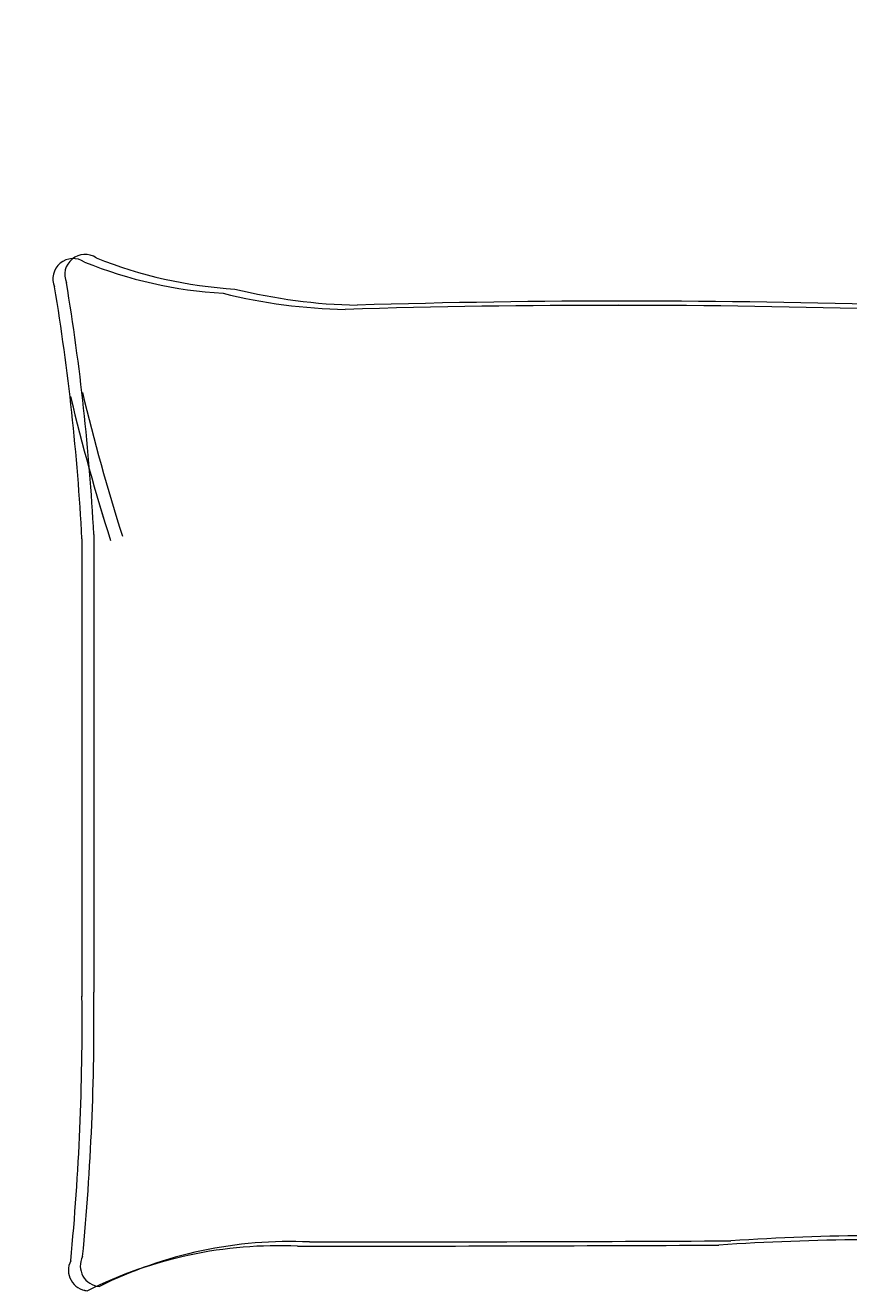
# Model space of a CAD drawing. Units: inches. Extents: x 1962 to 2771, y 1245 to 2660.
# Tile 73 of 114: x 2590 to 2626, y 2028 to 2082. Entities that reach past the tile are written whole.
import ezdxf

# ---------------------------------------------------------------- set-up
doc = ezdxf.new("R2010")
doc.units = ezdxf.units.IN
doc.layers.add('A-ANNO-DIMS', color=2, linetype='Continuous', lineweight=18)
doc.layers.add('A-FURN', color=8, linetype='Continuous', lineweight=13)
doc.styles.get("Standard").update_dxf_attribs({"font": 'arial.ttf'})
doc.dimstyles.get("Standard").update_dxf_attribs({"dimtxt": 0.18, "dimasz": 0.18, "dimexe": 0.18, "dimexo": 0.0625, "dimgap": 0.09, "dimtad": 0, "dimtih": 1, "dimtoh": 1, "dimdec": 4, "dimzin": 0, "dimdsep": 46, "dimtxsty": 'Standard', "dimcen": 0.09, "dimadec": 0, "dimazin": 0, "dimtfac": 1, "dimtdec": 4, "dimtofl": 0, "dimtmove": 0, "dimatfit": 3, "dimfxl": 1, "dimtolj": 1, "dimtzin": 0, "dimarcsym": 0})

# ---------------------------------------------------------------- blocks, each defined once
blk = doc.blocks.new('BED-PLAN')
for p, q in [((62.991, 11.975), (62.991, 31.54)), ((62.991, 11.975), (62.991, 31.54)), ((63.499, 12.157), (63.499, 31.722)), ((63.499, 12.156), (63.499, 31.722))]:
    blk.add_line(p, q)
for centre, radius, start, end in [((54.582, 60.538), 18.334, 267.4714, 296.4681), ((54.582, 60.538), 18.334, 267.4714, 296.4681), ((55.09, 60.719), 18.334, 267.4714, 296.4681), ((55.09, 60.719), 18.334, 267.4714, 296.4681), ((62.693, 43.251), 0.876, 332.6588, 86.02), ((62.693, 43.251), 0.876, 332.6588, 86.02), ((63.201, 43.433), 0.876, 332.6588, 86.02), ((63.201, 43.432), 0.876, 332.6588, 86.02), ((168.736, 32.712), 105.752, 174.4998, 180.63509), ((168.736, 32.712), 105.752, 174.4998, 180.63509), ((169.244, 32.894), 105.752, 174.4998, 180.63509), ((169.244, 32.894), 105.752, 174.4998, 180.63509), ((29.375, 145.064), 102.937, 266.97912, 273.83645), ((29.375, 145.063), 102.937, 266.97912, 273.83645), ((53.91, -3583.936), 3626.158, 90.002168, 90.286887), ((53.91, -3583.937), 3626.158, 90.002168, 90.286887), ((54.419, -3583.755), 3626.158, 90.002168, 90.286887), ((54.419, -3583.755), 3626.158, 90.002168, 90.286887), ((28.866, 144.882), 102.937, 266.97912, 273.83645), ((28.866, 144.882), 102.937, 266.97912, 273.83645), ((-18.848, -13.688), 84.623, 13.38322, 17.70533), ((-18.848, -13.688), 84.623, 13.38322, 17.70533), ((-18.34, -13.506), 84.623, 13.38322, 17.70533), ((-18.34, -13.507), 84.623, 13.38322, 17.70533), ((159.643, 17.033), 96.784, 182.99578, 189.40907), ((159.643, 17.033), 96.784, 182.99578, 189.40907), ((160.151, 17.215), 96.784, 182.99578, 189.40907), ((160.151, 17.215), 96.784, 182.99578, 189.40907), ((40.232, 385.38), 383.382, 268.22771, 271.71854), ((40.232, 385.38), 383.382, 268.22771, 271.71854), ((40.74, 385.562), 383.382, 268.22771, 271.71854), ((40.74, 385.561), 383.382, 268.22771, 271.71854), ((51.282, -21.381), 23.556, 76.0648, 88.9113), ((51.282, -21.381), 23.556, 76.0648, 88.9113), ((51.79, -21.199), 23.556, 76.0648, 88.9113), ((51.79, -21.199), 23.556, 76.0648, 88.9113), ((56.369, -17.034), 18.729, 67.9751, 86.652), ((56.369, -17.034), 18.729, 67.9751, 86.652), ((55.861, -17.215), 18.729, 67.9751, 86.652), ((55.861, -17.216), 18.729, 67.9751, 86.652), ((63.367, 0.866), 0.866, 236.1736, 23.4781), ((63.367, 0.866), 0.866, 236.1736, 23.4781), ((63.875, 1.047), 0.866, 236.1736, 23.4781), ((63.875, 1.047), 0.866, 236.1736, 23.4781)]:
    blk.add_arc(centre, radius, start, end)
blk = doc.blocks.new('*D40')
at = {"layer": 'A-ANNO-DIMS', "color": 0, "lineweight": -2, "transparency": 16777216}
for p, q in [((2072.02, 2033.906), (2072.02, 2583.474)), ((2072.2, 2583.294), (2366.02, 2583.294)), ((2660.627, 2583.294), (2366.808, 2583.294)), ((2660.807, 2524.406), (2660.807, 2583.474))]:
    blk.add_line(p, q, dxfattribs=at)
at = {"layer": 'A-ANNO-DIMS', "color": 0, "transparency": 16777216}
for points in [[(2072.2, 2583.324), (2072.2, 2583.264), (2072.02, 2583.294)], [(2660.627, 2583.324), (2660.627, 2583.264), (2660.807, 2583.294)]]:
    blk.add_solid(points, dxfattribs=at)
at = {"layer": 'Defpoints', "color": 0, "transparency": 16777216}
for p in [(2660.807, 2583.294), (2660.807, 2524.344), (2072.02, 2033.844)]:
    blk.add_point(p, dxfattribs=at)
at = {"layer": 'A-ANNO-DIMS', "color": 0, "transparency": 16777216, "insert": (2366.414, 2583.294), "char_height": 0.18, "attachment_point": 5}
blk.add_mtext('\\A1;588.8', dxfattribs=at)

msp = doc.modelspace()

# ---------------------------------------------------------------- block references
at = {"layer": 'A-FURN', "rotation": 180}
msp.add_blockref('BED-PLAN', (2656.3074, 2072.498), dxfattribs=at)

# ---------------------------------------------------------------- dimensions: what is measured, and where the dimension line sits
at = {"layer": 'A-ANNO-DIMS'}
dim = msp.add_linear_dim(base=(2660.8074, 2583.2937), p1=(2072.0204, 2033.8437), p2=(2660.8074, 2524.3437), dimstyle='Standard', override={"dimdec": 1, "dimlfac": 1, "dimrnd": 0, "dimzin": 0, "dimdsep": 46, "dimlunit": 2}, dxfattribs=at)
dim.commit()
dim.dimension.update_dxf_attribs({"geometry": '*D40', "text_midpoint": (2366.4139, 2583.2937)})

doc.saveas('drawing.dxf')
